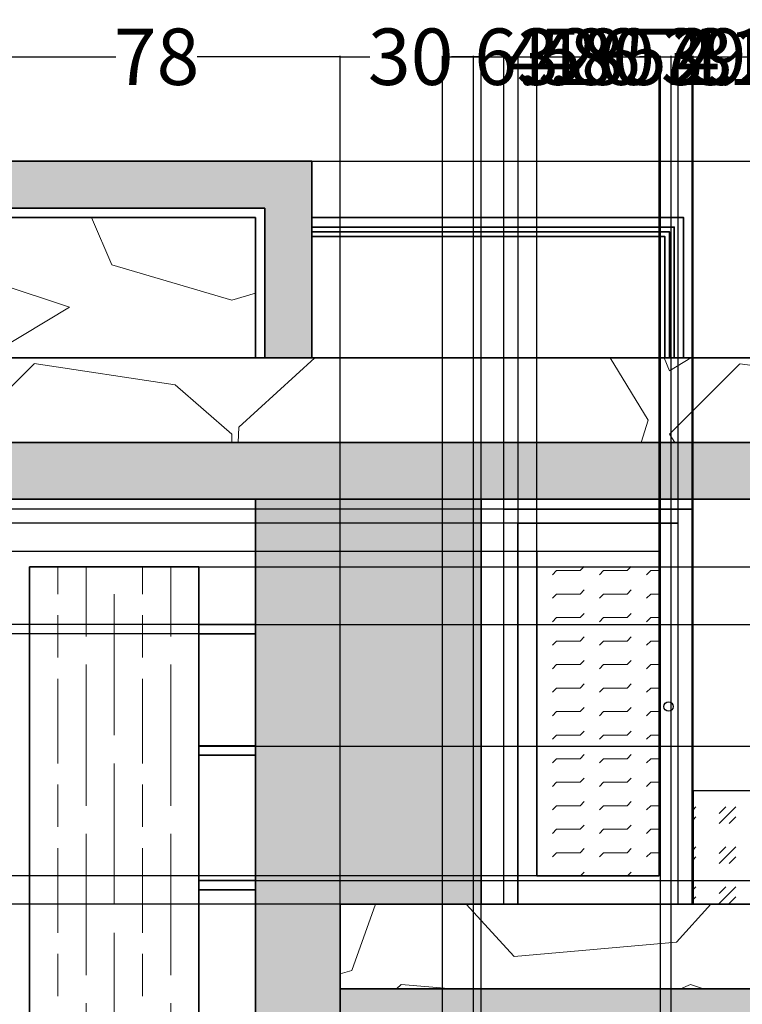
# Model space of a CAD drawing. Units: inches. Extents: x -73 to 458, y -161 to 332.
# Tile 4 of 6: x 106 to 259, y 123 to 332. Entities that reach past the tile are written whole.
import ezdxf

# ---------------------------------------------------------------- set-up
doc = ezdxf.new("R2010")
doc.units = ezdxf.units.IN
doc.header["$MEASUREMENT"] = 0
for name, color, linetype, lineweight in [('A-ANNO-DIMS', 2, 'Continuous', 18), ('A-DOOR', 4, 'Continuous', 25), ('A-ELEV', 7, 'Continuous', 35), ('A-ELEV-PATT', 8, 'Continuous', 13), ('A-GLAZ', 3, 'Continuous', 25), ('A-GLAZ-PATT', 8, 'Continuous', 13)]:
    doc.layers.add(name, color=color, linetype=linetype, lineweight=lineweight)
doc.styles.get("Standard").update_dxf_attribs({"font": 'arial.ttf'})
doc.dimstyles.get("Standard").update_dxf_attribs({"dimtxt": 12, "dimasz": 0.18, "dimexe": 0.18, "dimexo": 0.0625, "dimgap": 0.09, "dimtad": 0, "dimtih": 1, "dimtoh": 1, "dimdec": 0, "dimzin": 0, "dimdsep": 46, "dimlunit": 3, "dimtxsty": 'Standard', "dimcen": 0.09, "dimadec": 0, "dimazin": 0, "dimtfac": 1, "dimtdec": 0, "dimtofl": 0, "dimtmove": 0, "dimatfit": 3, "dimfxl": 1, "dimtolj": 1, "dimtzin": 0, "dimarcsym": 0})

# ---------------------------------------------------------------- blocks, each defined once
blk = doc.blocks.new('*U3')
blk.add_lwpolyline([(3.12, 0.01), (0.12, 0.01), (0.12, 84.01), (40.12, 84.01), (40.12, 0.01), (37.12, 0.01)])
for points in [[(37.12, 80.99), (37.12, 0.01), (3.12, 0.01), (3.12, 80.99)], [(33.12, 6.01), (33.12, 74.99), (7.12, 74.99), (7.12, 6.01)]]:
    blk.add_lwpolyline(points, close=True)
blk.add_circle((35.12, 42.01), 1)
blk = doc.blocks.new('*D6')
at = {"layer": 'A-ANNO-DIMS', "color": 0, "lineweight": -2, "transparency": 16777216}
for p, q in [((96, 260.27), (96, 324.4)), ((96.18, 324.22), (126.35, 324.22)), ((173.82, 324.22), (143.65, 324.22)), ((174, 126.13), (174, 324.4))]:
    blk.add_line(p, q, dxfattribs=at)
at = {"layer": 'A-ANNO-DIMS', "color": 0, "transparency": 16777216}
for points in [[(96.18, 324.25), (96.18, 324.19), (96, 324.22)], [(173.82, 324.25), (173.82, 324.19), (174, 324.22)]]:
    blk.add_solid(points, dxfattribs=at)
at = {"layer": 'Defpoints', "color": 0, "transparency": 16777216}
for p in [(174, 324.22), (96, 260.21), (174, 126.07)]:
    blk.add_point(p, dxfattribs=at)
at = {"layer": 'A-ANNO-DIMS', "color": 0, "transparency": 16777216, "insert": (135, 324.22), "char_height": 12, "attachment_point": 5}
blk.add_mtext('\\A1;78', dxfattribs=at)
blk = doc.blocks.new('*D7')
at = {"layer": 'A-ANNO-DIMS', "color": 0, "lineweight": -2, "transparency": 16777216}
for p, q in [((174, 126.13), (174, 324.4)), ((174.18, 324.22), (180.34, 324.22)), ((203.82, 324.22), (197.66, 324.22)), ((204, 24.13), (204, 324.4))]:
    blk.add_line(p, q, dxfattribs=at)
at = {"layer": 'A-ANNO-DIMS', "color": 0, "transparency": 16777216}
for points in [[(174.18, 324.25), (174.18, 324.19), (174, 324.22)], [(203.82, 324.25), (203.82, 324.19), (204, 324.22)]]:
    blk.add_solid(points, dxfattribs=at)
at = {"layer": 'Defpoints', "color": 0, "transparency": 16777216}
for p in [(204, 324.22), (174, 126.07), (204, 24.07)]:
    blk.add_point(p, dxfattribs=at)
at = {"layer": 'A-ANNO-DIMS', "color": 0, "transparency": 16777216, "insert": (189, 324.22), "char_height": 12, "attachment_point": 5}
blk.add_mtext('\\A1;30', dxfattribs=at)
blk = doc.blocks.new('*D8')
at = {"layer": 'A-ANNO-DIMS', "color": 0, "lineweight": -2, "transparency": 16777216}
for p, q in [((204, 24.13), (204, 324.4)), ((204.18, 324.22), (257.28, 324.22)), ((335.82, 324.22), (282.72, 324.22)), ((336, 126.13), (336, 324.4))]:
    blk.add_line(p, q, dxfattribs=at)
at = {"layer": 'A-ANNO-DIMS', "color": 0, "transparency": 16777216}
for points in [[(204.18, 324.25), (204.18, 324.19), (204, 324.22)], [(335.82, 324.25), (335.82, 324.19), (336, 324.22)]]:
    blk.add_solid(points, dxfattribs=at)
at = {"layer": 'Defpoints', "color": 0, "transparency": 16777216}
for p in [(336, 324.22), (336, 126.07), (204, 24.07)]:
    blk.add_point(p, dxfattribs=at)
at = {"layer": 'A-ANNO-DIMS', "color": 0, "transparency": 16777216, "insert": (270, 324.22), "char_height": 12, "attachment_point": 5}
blk.add_mtext('\\A1;132', dxfattribs=at)
blk = doc.blocks.new('*D25')
at = {"layer": 'A-ANNO-DIMS', "color": 0, "lineweight": -2, "transparency": 16777216}
for p, q in [((168.06, 302.02), (408.51, 302.02)), ((408.33, 301.84), (408.33, 287.33)), ((408.33, 260.39), (408.33, 274.9)), ((168.06, 260.21), (408.51, 260.21))]:
    blk.add_line(p, q, dxfattribs=at)
at = {"layer": 'A-ANNO-DIMS', "color": 0, "transparency": 16777216}
for points in [[(408.3, 301.84), (408.36, 301.84), (408.33, 302.02)], [(408.3, 260.39), (408.36, 260.39), (408.33, 260.21)]]:
    blk.add_solid(points, dxfattribs=at)
at = {"layer": 'Defpoints', "color": 0, "transparency": 16777216}
for p in [(168, 302.02), (408.33, 302.02), (168, 260.21)]:
    blk.add_point(p, dxfattribs=at)
at = {"layer": 'A-ANNO-DIMS', "color": 0, "transparency": 16777216, "insert": (408.33, 281.11), "char_height": 12, "attachment_point": 5}
blk.add_mtext('\\A1;41.814', dxfattribs=at)
blk = doc.blocks.new('*D42')
at = {"layer": 'A-ANNO-DIMS', "color": 0, "lineweight": -2, "transparency": 16777216}
for p, q in [((144.06, 149.14), (408.51, 149.14)), ((408.33, 148.96), (408.33, 140.32)), ((408.33, 119.24), (408.33, 127.88)), ((144.06, 119.06), (408.51, 119.06))]:
    blk.add_line(p, q, dxfattribs=at)
at = {"layer": 'A-ANNO-DIMS', "color": 0, "transparency": 16777216}
for points in [[(408.3, 148.96), (408.36, 148.96), (408.33, 149.14)], [(408.3, 119.24), (408.36, 119.24), (408.33, 119.06)]]:
    blk.add_solid(points, dxfattribs=at)
at = {"layer": 'Defpoints', "color": 0, "transparency": 16777216}
for p in [(144, 149.14), (408.33, 149.14), (144, 119.06)]:
    blk.add_point(p, dxfattribs=at)
at = {"layer": 'A-ANNO-DIMS', "color": 0, "transparency": 16777216, "insert": (408.33, 134.1), "char_height": 12, "attachment_point": 5}
blk.add_mtext('\\A1;30.08', dxfattribs=at)
blk = doc.blocks.new('*D43')
at = {"layer": 'A-ANNO-DIMS', "color": 0, "lineweight": -2, "transparency": 16777216}
for p, q in [((144.06, 177.7), (408.51, 177.7)), ((408.33, 177.52), (408.33, 169.64)), ((408.33, 149.32), (408.33, 157.2)), ((144.06, 149.14), (408.51, 149.14))]:
    blk.add_line(p, q, dxfattribs=at)
at = {"layer": 'A-ANNO-DIMS', "color": 0, "transparency": 16777216}
for points in [[(408.3, 177.52), (408.36, 177.52), (408.33, 177.7)], [(408.3, 149.32), (408.36, 149.32), (408.33, 149.14)]]:
    blk.add_solid(points, dxfattribs=at)
at = {"layer": 'Defpoints', "color": 0, "transparency": 16777216}
for p in [(144, 177.7), (408.33, 177.7), (144, 149.14)]:
    blk.add_point(p, dxfattribs=at)
at = {"layer": 'A-ANNO-DIMS', "color": 0, "transparency": 16777216, "insert": (408.33, 163.42), "char_height": 12, "attachment_point": 5}
blk.add_mtext('\\A1;28.57', dxfattribs=at)
blk = doc.blocks.new('*D44')
at = {"layer": 'A-ANNO-DIMS', "color": 0, "lineweight": -2, "transparency": 16777216}
for p, q in [((144.06, 203.54), (408.51, 203.54)), ((408.33, 203.36), (408.33, 196.84)), ((408.33, 177.88), (408.33, 184.4)), ((144.06, 177.7), (408.51, 177.7))]:
    blk.add_line(p, q, dxfattribs=at)
at = {"layer": 'A-ANNO-DIMS', "color": 0, "transparency": 16777216}
for points in [[(408.3, 203.36), (408.36, 203.36), (408.33, 203.54)], [(408.3, 177.88), (408.36, 177.88), (408.33, 177.7)]]:
    blk.add_solid(points, dxfattribs=at)
at = {"layer": 'Defpoints', "color": 0, "transparency": 16777216}
for p in [(144, 203.54), (408.33, 203.54), (144, 177.7)]:
    blk.add_point(p, dxfattribs=at)
at = {"layer": 'A-ANNO-DIMS', "color": 0, "transparency": 16777216, "insert": (408.33, 190.62), "char_height": 12, "attachment_point": 5}
blk.add_mtext('\\A1;25.83', dxfattribs=at)
blk = doc.blocks.new('*D45')
at = {"layer": 'A-ANNO-DIMS', "color": 0, "lineweight": -2, "transparency": 16777216}
for p, q in [((144.06, 215.8), (408.51, 215.8)), ((408.33, 215.8), (408.33, 215.98)), ((408.33, 215.98), (408.51, 215.98)), ((408.33, 203.72), (408.33, 215.62)), ((144.06, 203.54), (408.51, 203.54))]:
    blk.add_line(p, q, dxfattribs=at)
at = {"layer": 'A-ANNO-DIMS', "color": 0, "transparency": 16777216}
for points in [[(408.3, 215.62), (408.36, 215.62), (408.33, 215.8)], [(408.3, 203.72), (408.36, 203.72), (408.33, 203.54)]]:
    blk.add_solid(points, dxfattribs=at)
at = {"layer": 'Defpoints', "color": 0, "transparency": 16777216}
for p in [(144, 215.8), (408.33, 215.8), (144, 203.54)]:
    blk.add_point(p, dxfattribs=at)
at = {"layer": 'A-ANNO-DIMS', "color": 0, "transparency": 16777216, "insert": (432.98, 215.98), "char_height": 12, "attachment_point": 5}
blk.add_mtext('\\A1;12.265', dxfattribs=at)
blk = doc.blocks.new('*D46')
at = {"layer": 'A-ANNO-DIMS', "color": 0, "lineweight": -2, "transparency": 16777216}
for p, q in [((156.06, 230.21), (408.51, 230.21)), ((408.33, 230.03), (408.33, 229.22)), ((144.06, 215.8), (408.51, 215.8)), ((408.33, 215.98), (408.33, 216.79))]:
    blk.add_line(p, q, dxfattribs=at)
at = {"layer": 'A-ANNO-DIMS', "color": 0, "transparency": 16777216}
for points in [[(408.3, 230.03), (408.36, 230.03), (408.33, 230.21)], [(408.3, 215.98), (408.36, 215.98), (408.33, 215.8)]]:
    blk.add_solid(points, dxfattribs=at)
at = {"layer": 'Defpoints', "color": 0, "transparency": 16777216}
for p in [(156, 230.21), (408.33, 230.21), (144, 215.8)]:
    blk.add_point(p, dxfattribs=at)
at = {"layer": 'A-ANNO-DIMS', "color": 0, "transparency": 16777216, "insert": (408.33, 223), "char_height": 12, "attachment_point": 5}
blk.add_mtext('\\A1;14.406', dxfattribs=at)
blk = doc.blocks.new('*D47')
at = {"layer": 'A-ANNO-DIMS', "color": 0, "lineweight": -2, "transparency": 16777216}
for p, q in [((143.94, 203.54), (-41.78, 203.54)), ((-41.6, 203.36), (-41.6, 201.74)), ((143.94, 201.56), (-41.78, 201.56)), ((-41.6, 201.38), (-41.78, 201.38)), ((-41.6, 201.56), (-41.6, 201.38))]:
    blk.add_line(p, q, dxfattribs=at)
at = {"layer": 'A-ANNO-DIMS', "color": 0, "transparency": 16777216}
for points in [[(-41.63, 203.36), (-41.57, 203.36), (-41.6, 203.54)], [(-41.63, 201.74), (-41.57, 201.74), (-41.6, 201.56)]]:
    blk.add_solid(points, dxfattribs=at)
at = {"layer": 'Defpoints', "color": 0, "transparency": 16777216}
for p in [(144, 203.54), (-41.6, 201.56), (144, 201.56)]:
    blk.add_point(p, dxfattribs=at)
at = {"layer": 'A-ANNO-DIMS', "color": 0, "transparency": 16777216, "insert": (-56.91, 201.38), "char_height": 12, "attachment_point": 5}
blk.add_mtext('\\A1;1.98', dxfattribs=at)
blk = doc.blocks.new('*D48')
at = {"layer": 'A-ANNO-DIMS', "color": 0, "lineweight": -2, "transparency": 16777216}
for p, q in [((204, 144.13), (204, 324.4)), ((204.18, 324.22), (208.63, 324.22)), ((208.81, 144.14), (208.81, 324.4)), ((208.81, 324.22), (208.99, 324.22))]:
    blk.add_line(p, q, dxfattribs=at)
at = {"layer": 'A-ANNO-DIMS', "color": 0, "transparency": 16777216}
for points in [[(204.18, 324.25), (204.18, 324.19), (204, 324.22)], [(208.63, 324.25), (208.63, 324.19), (208.81, 324.22)]]:
    blk.add_solid(points, dxfattribs=at)
at = {"layer": 'Defpoints', "color": 0, "transparency": 16777216}
for p in [(208.81, 324.22), (204, 144.07), (208.81, 144.08)]:
    blk.add_point(p, dxfattribs=at)
at = {"layer": 'A-ANNO-DIMS', "color": 0, "transparency": 16777216, "insert": (229.56, 324.22), "char_height": 12, "attachment_point": 5}
blk.add_mtext('\\A1;4.807', dxfattribs=at)
blk = doc.blocks.new('*D49')
at = {"layer": 'A-ANNO-DIMS', "color": 0, "lineweight": -2, "transparency": 16777216}
for p, q in [((208.81, 144.14), (208.81, 324.4)), ((208.99, 324.22), (211.63, 324.22)), ((211.81, 144.14), (211.81, 324.4)), ((211.81, 324.22), (211.99, 324.22))]:
    blk.add_line(p, q, dxfattribs=at)
at = {"layer": 'A-ANNO-DIMS', "color": 0, "transparency": 16777216}
for points in [[(208.99, 324.25), (208.99, 324.19), (208.81, 324.22)], [(211.63, 324.25), (211.63, 324.19), (211.81, 324.22)]]:
    blk.add_solid(points, dxfattribs=at)
at = {"layer": 'Defpoints', "color": 0, "transparency": 16777216}
for p in [(211.81, 324.22), (208.81, 144.08), (211.81, 144.08)]:
    blk.add_point(p, dxfattribs=at)
at = {"layer": 'A-ANNO-DIMS', "color": 0, "transparency": 16777216, "insert": (216, 324.22), "char_height": 12, "attachment_point": 5}
blk.add_mtext('\\A1;3', dxfattribs=at)
blk = doc.blocks.new('*D50')
at = {"layer": 'A-ANNO-DIMS', "color": 0, "lineweight": -2, "transparency": 16777216}
for p, q in [((211.81, 144.14), (211.81, 324.4)), ((211.99, 324.22), (215.63, 324.22)), ((215.81, 150.14), (215.81, 324.4)), ((215.81, 324.22), (215.99, 324.22))]:
    blk.add_line(p, q, dxfattribs=at)
at = {"layer": 'A-ANNO-DIMS', "color": 0, "transparency": 16777216}
for points in [[(211.99, 324.25), (211.99, 324.19), (211.81, 324.22)], [(215.63, 324.25), (215.63, 324.19), (215.81, 324.22)]]:
    blk.add_solid(points, dxfattribs=at)
at = {"layer": 'Defpoints', "color": 0, "transparency": 16777216}
for p in [(215.81, 324.22), (215.81, 150.08), (211.81, 144.08)]:
    blk.add_point(p, dxfattribs=at)
at = {"layer": 'A-ANNO-DIMS', "color": 0, "transparency": 16777216, "insert": (220.23, 324.22), "char_height": 12, "attachment_point": 5}
blk.add_mtext('\\A1;4', dxfattribs=at)
blk = doc.blocks.new('*D51')
at = {"layer": 'A-ANNO-DIMS', "color": 0, "lineweight": -2, "transparency": 16777216}
for p, q in [((215.81, 150.14), (215.81, 324.4)), ((215.99, 324.22), (220.02, 324.22)), ((241.63, 324.22), (237.59, 324.22)), ((241.81, 150.14), (241.81, 324.4))]:
    blk.add_line(p, q, dxfattribs=at)
at = {"layer": 'A-ANNO-DIMS', "color": 0, "transparency": 16777216}
for points in [[(215.99, 324.25), (215.99, 324.19), (215.81, 324.22)], [(241.63, 324.25), (241.63, 324.19), (241.81, 324.22)]]:
    blk.add_solid(points, dxfattribs=at)
at = {"layer": 'Defpoints', "color": 0, "transparency": 16777216}
for p in [(241.81, 324.22), (215.81, 150.08), (241.81, 150.08)]:
    blk.add_point(p, dxfattribs=at)
at = {"layer": 'A-ANNO-DIMS', "color": 0, "transparency": 16777216, "insert": (228.81, 324.22), "char_height": 12, "attachment_point": 5}
blk.add_mtext('\\A1;26', dxfattribs=at)
blk = doc.blocks.new('*D52')
at = {"layer": 'A-ANNO-DIMS', "color": 0, "lineweight": -2, "transparency": 16777216}
for p, q in [((241.81, 150.14), (241.81, 324.4)), ((241.99, 324.22), (245.63, 324.22)), ((245.81, 144.14), (245.81, 324.4)), ((245.81, 324.22), (245.99, 324.22))]:
    blk.add_line(p, q, dxfattribs=at)
at = {"layer": 'A-ANNO-DIMS', "color": 0, "transparency": 16777216}
for points in [[(241.99, 324.25), (241.99, 324.19), (241.81, 324.22)], [(245.63, 324.25), (245.63, 324.19), (245.81, 324.22)]]:
    blk.add_solid(points, dxfattribs=at)
at = {"layer": 'Defpoints', "color": 0, "transparency": 16777216}
for p in [(245.81, 324.22), (241.81, 150.08), (245.81, 144.08)]:
    blk.add_point(p, dxfattribs=at)
at = {"layer": 'A-ANNO-DIMS', "color": 0, "transparency": 16777216, "insert": (250.23, 324.22), "char_height": 12, "attachment_point": 5}
blk.add_mtext('\\A1;4', dxfattribs=at)
blk = doc.blocks.new('*D53')
at = {"layer": 'A-ANNO-DIMS', "color": 0, "lineweight": -2, "transparency": 16777216}
for p, q in [((245.81, 144.14), (245.81, 324.4)), ((245.99, 324.22), (248.63, 324.22)), ((248.81, 144.14), (248.81, 324.4)), ((248.81, 324.22), (248.99, 324.22))]:
    blk.add_line(p, q, dxfattribs=at)
at = {"layer": 'A-ANNO-DIMS', "color": 0, "transparency": 16777216}
for points in [[(245.99, 324.25), (245.99, 324.19), (245.81, 324.22)], [(248.63, 324.25), (248.63, 324.19), (248.81, 324.22)]]:
    blk.add_solid(points, dxfattribs=at)
at = {"layer": 'Defpoints', "color": 0, "transparency": 16777216}
for p in [(248.81, 324.22), (245.81, 144.08), (248.81, 144.08)]:
    blk.add_point(p, dxfattribs=at)
at = {"layer": 'A-ANNO-DIMS', "color": 0, "transparency": 16777216, "insert": (253, 324.22), "char_height": 12, "attachment_point": 5}
blk.add_mtext('\\A1;3', dxfattribs=at)
blk = doc.blocks.new('*D54')
at = {"layer": 'A-ANNO-DIMS', "color": 0, "lineweight": -2, "transparency": 16777216}
for p, q in [((249, 168.25), (249, 324.4)), ((249.18, 324.22), (262.15, 324.22)), ((262.33, 168.25), (262.33, 324.4)), ((262.33, 324.22), (262.51, 324.22))]:
    blk.add_line(p, q, dxfattribs=at)
at = {"layer": 'A-ANNO-DIMS', "color": 0, "transparency": 16777216}
for points in [[(249.18, 324.25), (249.18, 324.19), (249, 324.22)], [(262.15, 324.25), (262.15, 324.19), (262.33, 324.22)]]:
    blk.add_solid(points, dxfattribs=at)
at = {"layer": 'Defpoints', "color": 0, "transparency": 16777216}
for p in [(262.33, 324.22), (249, 168.19), (262.33, 168.19)]:
    blk.add_point(p, dxfattribs=at)
at = {"layer": 'A-ANNO-DIMS', "color": 0, "transparency": 16777216, "insert": (282.28, 324.22), "char_height": 12, "attachment_point": 5}
blk.add_mtext('\\A1;13.33', dxfattribs=at)
blk = doc.blocks.new('*D61')
at = {"layer": 'A-ANNO-DIMS', "color": 0, "lineweight": -2, "transparency": 16777216}
for p, q in [((241.74, 150.08), (-41.78, 150.08)), ((-41.6, 150.08), (-41.6, 150.26)), ((-41.6, 150.26), (-41.42, 150.26)), ((-41.6, 144.26), (-41.6, 149.9)), ((248.74, 144.08), (-41.78, 144.08))]:
    blk.add_line(p, q, dxfattribs=at)
at = {"layer": 'A-ANNO-DIMS', "color": 0, "transparency": 16777216}
for points in [[(-41.63, 149.9), (-41.57, 149.9), (-41.6, 150.08)], [(-41.63, 144.26), (-41.57, 144.26), (-41.6, 144.08)]]:
    blk.add_solid(points, dxfattribs=at)
at = {"layer": 'Defpoints', "color": 0, "transparency": 16777216}
for p in [(-41.6, 150.08), (241.81, 150.08), (248.81, 144.08)]:
    blk.add_point(p, dxfattribs=at)
at = {"layer": 'A-ANNO-DIMS', "color": 0, "transparency": 16777216, "insert": (-37.37, 150.26), "char_height": 12, "attachment_point": 5}
blk.add_mtext('\\A1;6', dxfattribs=at)
blk = doc.blocks.new('*D62')
at = {"layer": 'A-ANNO-DIMS', "color": 0, "lineweight": -2, "transparency": 16777216}
for p, q in [((241.74, 219.06), (-41.78, 219.06)), ((-41.6, 218.88), (-41.6, 190.78)), ((-41.6, 150.26), (-41.6, 178.35)), ((241.74, 150.08), (-41.78, 150.08))]:
    blk.add_line(p, q, dxfattribs=at)
at = {"layer": 'A-ANNO-DIMS', "color": 0, "transparency": 16777216}
for points in [[(-41.63, 218.88), (-41.57, 218.88), (-41.6, 219.06)], [(-41.63, 150.26), (-41.57, 150.26), (-41.6, 150.08)]]:
    blk.add_solid(points, dxfattribs=at)
at = {"layer": 'Defpoints', "color": 0, "transparency": 16777216}
for p in [(-41.6, 219.06), (241.81, 219.06), (241.81, 150.08)]:
    blk.add_point(p, dxfattribs=at)
at = {"layer": 'A-ANNO-DIMS', "color": 0, "transparency": 16777216, "insert": (-41.6, 184.57), "char_height": 12, "attachment_point": 5}
blk.add_mtext('\\A1;68.98', dxfattribs=at)
blk = doc.blocks.new('*D63')
at = {"layer": 'A-ANNO-DIMS', "color": 0, "lineweight": -2, "transparency": 16777216}
for p, q in [((245.74, 225.06), (-41.78, 225.06)), ((-41.6, 225.06), (-41.6, 225.24)), ((-41.6, 225.24), (-41.42, 225.24)), ((-41.6, 219.24), (-41.6, 224.88)), ((241.74, 219.06), (-41.78, 219.06))]:
    blk.add_line(p, q, dxfattribs=at)
at = {"layer": 'A-ANNO-DIMS', "color": 0, "transparency": 16777216}
for points in [[(-41.63, 224.88), (-41.57, 224.88), (-41.6, 225.06)], [(-41.63, 219.24), (-41.57, 219.24), (-41.6, 219.06)]]:
    blk.add_solid(points, dxfattribs=at)
at = {"layer": 'Defpoints', "color": 0, "transparency": 16777216}
for p in [(-41.6, 225.06), (245.81, 225.06), (241.81, 219.06)]:
    blk.add_point(p, dxfattribs=at)
at = {"layer": 'A-ANNO-DIMS', "color": 0, "transparency": 16777216, "insert": (-37.37, 225.24), "char_height": 12, "attachment_point": 5}
blk.add_mtext('\\A1;6', dxfattribs=at)
blk = doc.blocks.new('*D64')
at = {"layer": 'A-ANNO-DIMS', "color": 0, "lineweight": -2, "transparency": 16777216}
for p, q in [((-41.6, 228.08), (-41.6, 228.26)), ((-41.6, 228.26), (-41.42, 228.26)), ((248.74, 228.08), (-41.78, 228.08)), ((-41.6, 225.24), (-41.6, 227.9)), ((245.74, 225.06), (-41.78, 225.06))]:
    blk.add_line(p, q, dxfattribs=at)
at = {"layer": 'A-ANNO-DIMS', "color": 0, "transparency": 16777216}
for points in [[(-41.63, 227.9), (-41.57, 227.9), (-41.6, 228.08)], [(-41.63, 225.24), (-41.57, 225.24), (-41.6, 225.06)]]:
    blk.add_solid(points, dxfattribs=at)
at = {"layer": 'Defpoints', "color": 0, "transparency": 16777216}
for p in [(-41.6, 228.08), (248.81, 228.08), (245.81, 225.06)]:
    blk.add_point(p, dxfattribs=at)
at = {"layer": 'A-ANNO-DIMS', "color": 0, "transparency": 16777216, "insert": (-21.09, 228.26), "char_height": 12, "attachment_point": 5}
blk.add_mtext('\\A1;3.023', dxfattribs=at)
blk = doc.blocks.new('*D71')
at = {"layer": 'A-ANNO-DIMS', "color": 0, "lineweight": -2, "transparency": 16777216}
for p, q in [((195.77, -5.87), (195.77, 324.4)), ((195.95, 324.22), (202.17, 324.22)), ((202.35, -5.87), (202.35, 324.4)), ((202.35, 324.22), (202.53, 324.22))]:
    blk.add_line(p, q, dxfattribs=at)
at = {"layer": 'A-ANNO-DIMS', "color": 0, "transparency": 16777216}
for points in [[(195.95, 324.25), (195.95, 324.19), (195.77, 324.22)], [(202.17, 324.25), (202.17, 324.19), (202.35, 324.22)]]:
    blk.add_solid(points, dxfattribs=at)
at = {"layer": 'Defpoints', "color": 0, "transparency": 16777216}
for p in [(202.35, 324.22), (195.77, -5.93), (202.35, -5.93)]:
    blk.add_point(p, dxfattribs=at)
at = {"layer": 'A-ANNO-DIMS', "color": 0, "transparency": 16777216, "insert": (222.95, 324.22), "char_height": 12, "attachment_point": 5}
blk.add_mtext('\\A1;6.585', dxfattribs=at)
blk = doc.blocks.new('*D72')
at = {"layer": 'A-ANNO-DIMS', "color": 0, "lineweight": -2, "transparency": 16777216}
for p, q in [((202.35, -5.87), (202.35, 324.4)), ((202.53, 324.22), (241.93, 324.22)), ((242.11, -5.87), (242.11, 324.4)), ((242.11, 324.22), (242.29, 324.22))]:
    blk.add_line(p, q, dxfattribs=at)
at = {"layer": 'A-ANNO-DIMS', "color": 0, "transparency": 16777216}
for points in [[(202.53, 324.25), (202.53, 324.19), (202.35, 324.22)], [(241.93, 324.25), (241.93, 324.19), (242.11, 324.22)]]:
    blk.add_solid(points, dxfattribs=at)
at = {"layer": 'Defpoints', "color": 0, "transparency": 16777216}
for p in [(242.11, 324.22), (202.35, -5.93), (242.11, -5.93)]:
    blk.add_point(p, dxfattribs=at)
at = {"layer": 'A-ANNO-DIMS', "color": 0, "transparency": 16777216, "insert": (262.62, 324.22), "char_height": 12, "attachment_point": 5}
blk.add_mtext('\\A1;39.76', dxfattribs=at)
blk = doc.blocks.new('*D73')
at = {"layer": 'A-ANNO-DIMS', "color": 0, "lineweight": -2, "transparency": 16777216}
for p, q in [((242.11, -5.87), (242.11, 324.4)), ((242.29, 324.22), (244.17, 324.22)), ((244.35, -5.87), (244.35, 324.4)), ((244.35, 324.22), (244.53, 324.22))]:
    blk.add_line(p, q, dxfattribs=at)
at = {"layer": 'A-ANNO-DIMS', "color": 0, "transparency": 16777216}
for points in [[(242.29, 324.25), (242.29, 324.19), (242.11, 324.22)], [(244.17, 324.25), (244.17, 324.19), (244.35, 324.22)]]:
    blk.add_solid(points, dxfattribs=at)
at = {"layer": 'Defpoints', "color": 0, "transparency": 16777216}
for p in [(244.35, 324.22), (242.11, -5.93), (244.35, -5.93)]:
    blk.add_point(p, dxfattribs=at)
at = {"layer": 'A-ANNO-DIMS', "color": 0, "transparency": 16777216, "insert": (264.95, 324.22), "char_height": 12, "attachment_point": 5}
blk.add_mtext('\\A1;2.244', dxfattribs=at)
blk = doc.blocks.new('*D74')
at = {"layer": 'A-ANNO-DIMS', "color": 0, "lineweight": -2, "transparency": 16777216}
for p, q in [((244.35, -5.87), (244.35, 324.4)), ((244.53, 324.22), (277.93, 324.22)), ((278.11, -5.87), (278.11, 324.4)), ((278.11, 324.22), (278.29, 324.22))]:
    blk.add_line(p, q, dxfattribs=at)
at = {"layer": 'A-ANNO-DIMS', "color": 0, "transparency": 16777216}
for points in [[(244.53, 324.25), (244.53, 324.19), (244.35, 324.22)], [(277.93, 324.25), (277.93, 324.19), (278.11, 324.22)]]:
    blk.add_solid(points, dxfattribs=at)
at = {"layer": 'Defpoints', "color": 0, "transparency": 16777216}
for p in [(278.11, 324.22), (244.35, -5.93), (278.11, -5.93)]:
    blk.add_point(p, dxfattribs=at)
at = {"layer": 'A-ANNO-DIMS', "color": 0, "transparency": 16777216, "insert": (303.28, 324.22), "char_height": 12, "attachment_point": 5}
blk.add_mtext('\\A1;33.756', dxfattribs=at)

msp = doc.modelspace()

# ---------------------------------------------------------------- hatches: boundary and pattern name
at = {"layer": 'A-ELEV-PATT'}
h = msp.add_hatch(color=256, dxfattribs=at)
h.dxf.hatch_style = 1
h.paths.add_polyline_path([(167.9979, 302.0202), (155.9979, 302.0202), (95.9979, 302.0202), (23.9979, 302.0202), (23.9979, -113.9335), (33.9979, -113.9335), (33.9979, 292.0202), (95.9979, 292.0202), (157.9979, 292.0202), (157.9979, 260.2059), (167.9979, 260.2059), (167.9979, 290.0202)])
h.paths.add_polyline_path([(335.9979, 242.2059), (323.9979, 242.2059), (95.9979, 242.2059), (95.9979, 234.0665), (95.9979, 230.2059), (323.9979, 230.2059), (335.9979, 230.2059)])
h.paths.add_polyline_path([(335.9979, 126.0665), (323.9979, 126.0665), (173.9979, 126.0665), (173.9979, 114.0665), (323.9979, 114.0665), (335.9979, 114.0665)])
h.paths.add_polyline_path([(335.9979, 6.0665), (323.9979, 6.0665), (95.9979, 6.0665), (95.9979, -5.9335), (323.9979, -5.9335), (335.9979, -5.9335)])
h = msp.add_hatch(dxfattribs=at)
h.set_pattern_fill('GRAVEL', color=256, scale=150)
h.paths.add_polyline_path([(95.9979, 234.0665), (95.9979, 260.2059), (155.9979, 260.2059), (155.9979, 290.0202), (95.9979, 290.0202), (55.9979, 290.0202), (55.9979, -113.9335), (95.9979, -113.9335), (95.9979, 24.0665), (95.9979, 54.0267)])
h.paths.add_polyline_path([(323.9979, 144.0665), (248.9979, 144.0665), (173.9979, 144.0665), (173.9979, 126.0665), (323.9979, 126.0665)])
h.paths.add_polyline_path([(323.9979, 24.0665), (248.9979, 24.0665), (155.9979, 24.0665), (155.9979, 6.0665), (323.9979, 6.0665)])
h.paths.add_polyline_path([(323.9979, 260.2059), (95.9979, 260.2059), (95.9979, 242.2059), (323.9979, 242.2059)])
h.paths.add_polyline_path([(155.9979, 24.0665), (95.9979, 24.0665), (95.9979, 6.0665), (155.9979, 6.0665)], flags=17)
h = msp.add_hatch(color=256, dxfattribs=at)
h.dxf.hatch_style = 1
h.paths.add_polyline_path([(195.7666, -5.9335), (155.3839, -5.9335), (155.3839, -113.9335), (195.7666, -113.9335)])
h.paths.add_polyline_path([(323.9979, -5.9335), (284.4845, -5.9335), (284.4845, -113.9335), (323.9979, -113.9335)])
h.paths.add_polyline_path([(203.9979, 114.0665), (173.9979, 114.0665), (173.9979, 144.0665), (203.9979, 144.0665), (203.9979, 230.2059), (155.9979, 230.2059), (155.9979, 24.0665), (203.9979, 24.0665)])
h = msp.add_hatch(dxfattribs=at)
h.set_pattern_fill('FLEX', color=256, scale=20)
h.paths.add_polyline_path([(241.805, 219.0563), (215.805, 219.0563), (215.805, 150.0793), (241.805, 150.0793)])
h.paths.add_polyline_path([(241.805, 99.0563), (215.805, 99.0563), (215.805, 30.0793), (241.805, 30.0793)])
h.paths.add_polyline_path([(138.915, -38.9437), (112.915, -38.9437), (112.915, -107.9207), (138.915, -107.9207)])
h = msp.add_hatch(dxfattribs=at)
h.set_pattern_fill('GOST_WOOD', color=256, scale=3)
h.set_pattern_definition([(90, (0, 0), (18, -1e-15), [30, -6]), (90, (6, -6), (18, -1e-15), [18, -4.5, 9, -4.5]), (90, (12, -15), (18, -1e-15), [30, -6])])
h.paths.add_polyline_path([(143.9979, 215.8003), (107.9979, 215.8003), (107.9979, 54.0267), (143.9979, 54.0267)])

# ---------------------------------------------------------------- linework, layer by layer
at = {"layer": 'A-ELEV'}
for p, q in [((167.9979, 260.2059), (167.9979, 290.0202)), ((323.9979, 260.2059), (95.9979, 260.2059)), ((246.9957, 260.2059), (167.9979, 260.2059)), ((323.9979, 242.2059), (95.9979, 242.2059)), ((323.9979, 230.2059), (95.9979, 230.2059)), ((155.9979, 6.0665), (155.9979, 230.2059)), ((203.9979, 144.0665), (203.9979, 230.2059)), ((107.9979, 215.8003), (107.9979, 54.0267)), ((143.9979, 215.8003), (107.9979, 215.8003)), ((143.9979, 54.0267), (143.9979, 215.8003)), ((323.9979, 144.0665), (173.9979, 144.0665)), ((173.9979, 144.0665), (173.9979, 114.0665)), ((323.9979, 126.0665), (173.9979, 126.0665))]:
    msp.add_line(p, q, dxfattribs=at)
for points in [[(167.9979, 260.2059), (167.9979, 302.0202), (155.9979, 302.0202), (95.9979, 302.0202), (23.9979, 302.0202), (23.9979, -113.9335)], [(157.9979, 260.2059), (157.9979, 292.0202), (95.9979, 292.0202), (33.9979, 292.0202), (33.9979, -113.9335)], [(155.9979, 260.2059), (155.9979, 290.0202), (95.9979, 290.0202), (35.9979, 290.0202), (35.9979, -113.9335)], [(167.9979, 290.0202), (246.9957, 290.0202), (246.9957, 260.2059)], [(167.9979, 288.0202), (244.9957, 288.0202), (244.9957, 260.2059)], [(167.9979, 287.0202), (243.9957, 287.0202), (243.9957, 260.2059)], [(167.9979, 286.0202), (242.9957, 286.0202), (242.9957, 260.2059)]]:
    msp.add_lwpolyline(points, dxfattribs=at)
for points in [[(143.9979, 203.5354), (155.9979, 203.5354), (155.9979, 201.5578), (143.9979, 201.5578)], [(143.9979, 177.7045), (155.9979, 177.7045), (155.9979, 175.727), (143.9979, 175.727)], [(143.9979, 149.136), (155.9979, 149.136), (155.9979, 147.1585), (143.9979, 147.1585)]]:
    msp.add_lwpolyline(points, close=True, dxfattribs=at)
at = {"layer": 'A-GLAZ'}
msp.add_lwpolyline([(248.9979, 144.0665), (323.9979, 144.0665), (323.9979, 168.1912), (248.9979, 168.1912)], close=True, dxfattribs=at)
at = {"layer": 'A-GLAZ-PATT'}
for p, q in [((248.9979, 164.145), (249.6087, 164.7559)), ((254.5584, 161.2203), (258.094, 164.7559)), ((254.5584, 163.3417), (255.9727, 164.7559)), ((248.9979, 162.0237), (249.6087, 162.6346)), ((256.6798, 161.2203), (258.094, 162.6346)), ((248.9979, 155.6598), (249.6087, 156.2706)), ((254.5584, 152.7351), (258.094, 156.2706)), ((254.5584, 154.8564), (255.9727, 156.2706)), ((248.9979, 153.5384), (249.6087, 154.1493)), ((256.6798, 152.7351), (258.094, 154.1493)), ((248.9979, 147.1745), (249.6087, 147.7853)), ((254.5584, 144.2498), (258.094, 147.7853)), ((254.5584, 146.3711), (255.9727, 147.7853)), ((248.9979, 145.0532), (249.6087, 145.664)), ((256.6798, 144.2498), (258.094, 145.664))]:
    msp.add_line(p, q, dxfattribs=at)

# ---------------------------------------------------------------- block references
at = {"layer": 'A-DOOR'}
msp.add_blockref('*U3', (208.6813, 144.0665), dxfattribs=at)

# ---------------------------------------------------------------- dimensions: what is measured, and where the dimension line sits
at = {"layer": 'A-ANNO-DIMS'}
for base, p1, p2, override, picture, middle in [((173.9979, 324.2202), (95.9979, 260.2059), (173.9979, 126.0665), {"dimdec": 0, "dimlfac": 1, "dimrnd": 0, "dimzin": 0, "dimdsep": 46, "dimlunit": 2}, '*D6', (134.9979, 324.2202)), ((203.9979, 324.2202), (173.9979, 126.0665), (203.9979, 24.0665), {"dimdec": 0, "dimlfac": 1, "dimrnd": 0, "dimzin": 0, "dimdsep": 46, "dimlunit": 2}, '*D7', (188.9979, 324.2202)), ((202.3513, 324.2202), (195.7666, -5.9335), (202.3513, -5.9335), {"dimdec": 3, "dimlfac": 1, "dimrnd": 0, "dimzin": 0, "dimdsep": 46, "dimlunit": 2}, '*D71', (222.946, 324.2202)), ((242.1074, 324.2202), (202.3513, -5.9335), (242.1074, -5.9335), {"dimdec": 2, "dimlfac": 1, "dimrnd": 0, "dimzin": 0, "dimdsep": 46, "dimlunit": 2}, '*D72', (262.6161, 324.2202)), ((335.9979, 324.2202), (203.9979, 24.0665), (335.9979, 126.0665), {"dimdec": 0, "dimlfac": 1, "dimrnd": 0, "dimzin": 0, "dimdsep": 46, "dimlunit": 2}, '*D8', (269.9979, 324.2202)), ((208.805, 324.2202), (203.9979, 144.0665), (208.805, 144.0793), {"dimdec": 3, "dimlfac": 1, "dimrnd": 0, "dimzin": 0, "dimdsep": 46, "dimlunit": 2}, '*D48', (229.5634, 324.2202)), ((211.805, 324.2202), (208.805, 144.0793), (211.805, 144.0793), {"dimdec": 0, "dimlfac": 1, "dimrnd": 0, "dimzin": 0, "dimdsep": 46, "dimlunit": 2}, '*D49', (216.0041, 324.2202)), ((215.805, 324.2202), (211.805, 144.0793), (215.805, 150.0793), {"dimdec": 0, "dimlfac": 1, "dimrnd": 0, "dimzin": 0, "dimdsep": 46, "dimlunit": 2}, '*D50', (220.2251, 324.2202)), ((241.805, 324.2202), (215.805, 150.0793), (241.805, 150.0793), {"dimdec": 0, "dimlfac": 1, "dimrnd": 0, "dimzin": 0, "dimdsep": 46, "dimlunit": 2}, '*D51', (228.805, 324.2202)), ((245.805, 324.2202), (241.805, 150.0793), (245.805, 144.0793), {"dimdec": 0, "dimlfac": 1, "dimrnd": 0, "dimzin": 0, "dimdsep": 46, "dimlunit": 2}, '*D52', (250.2251, 324.2202)), ((244.3513, 324.2202), (242.1074, -5.9335), (244.3513, -5.9335), {"dimdec": 3, "dimlfac": 1, "dimrnd": 0, "dimzin": 0, "dimdsep": 46, "dimlunit": 2}, '*D73', (264.946, 324.2202)), ((278.1074, 324.2202), (244.3513, -5.9335), (278.1074, -5.9335), {"dimdec": 3, "dimlfac": 1, "dimrnd": 0, "dimzin": 0, "dimdsep": 46, "dimlunit": 2}, '*D74', (303.2778, 324.2202)), ((248.805, 324.2202), (245.805, 144.0793), (248.805, 144.0793), {"dimdec": 0, "dimlfac": 1, "dimrnd": 0, "dimzin": 0, "dimdsep": 46, "dimlunit": 2}, '*D53', (253.0041, 324.2202)), ((262.3267, 324.2202), (248.9979, 168.1912), (262.3267, 168.1912), {"dimdec": 2, "dimlfac": 1, "dimrnd": 0, "dimzin": 0, "dimdsep": 46, "dimlunit": 2}, '*D54', (282.2788, 324.2202))]:
    dim = msp.add_linear_dim(base=base, p1=p1, p2=p2, dimstyle='Standard', override=override, dxfattribs=at)
    dim.commit()
    dim.dimension.update_dxf_attribs({"geometry": picture, "text_midpoint": middle})
for base, p1, p2, override, picture, middle in [((408.326, 302.0202), (167.9979, 260.2059), (167.9979, 302.0202), {"dimdec": 3, "dimlfac": 1, "dimrnd": 0, "dimzin": 0, "dimdsep": 46, "dimlunit": 2}, '*D25', (408.326, 281.1131)), ((-41.6031, 228.0793), (245.805, 225.0563), (248.805, 228.0793), {"dimdec": 3, "dimlfac": 1, "dimrnd": 0, "dimzin": 0, "dimdsep": 46, "dimlunit": 2}, '*D64', (-21.0903, 228.2593)), ((-41.6031, 225.0563), (241.805, 219.0563), (245.805, 225.0563), {"dimdec": 0, "dimlfac": 1, "dimrnd": 0, "dimzin": 0, "dimdsep": 46, "dimlunit": 2}, '*D63', (-37.3713, 225.2363)), ((408.326, 230.2059), (143.9979, 215.8003), (155.9979, 230.2059), {"dimdec": 3, "dimlfac": 1, "dimrnd": 0, "dimzin": 0, "dimdsep": 46, "dimlunit": 2}, '*D46', (408.326, 223.0031)), ((408.326, 215.8003), (143.9979, 203.5354), (143.9979, 215.8003), {"dimdec": 3, "dimlfac": 1, "dimrnd": 0, "dimzin": 0, "dimdsep": 46, "dimlunit": 2}, '*D45', (432.9848, 215.9803)), ((-41.6031, 219.0563), (241.805, 150.0793), (241.805, 219.0563), {"dimdec": 2, "dimlfac": 1, "dimrnd": 0, "dimzin": 0, "dimdsep": 46, "dimlunit": 2}, '*D62', (-41.6031, 184.5678)), ((-41.6031, 201.5578), (143.9979, 203.5354), (143.9979, 201.5578), {"dimdec": 2, "dimlfac": 1, "dimrnd": 0, "dimzin": 0, "dimdsep": 46, "dimlunit": 2}, '*D47', (-56.9059, 201.3778)), ((408.326, 203.5354), (143.9979, 177.7045), (143.9979, 203.5354), {"dimdec": 2, "dimlfac": 1, "dimrnd": 0, "dimzin": 0, "dimdsep": 46, "dimlunit": 2}, '*D44', (408.326, 190.6199)), ((408.326, 177.7045), (143.9979, 149.136), (143.9979, 177.7045), {"dimdec": 2, "dimlfac": 1, "dimrnd": 0, "dimzin": 0, "dimdsep": 46, "dimlunit": 2}, '*D43', (408.326, 163.4203)), ((-41.6031, 150.0793), (248.805, 144.0793), (241.805, 150.0793), {"dimdec": 0, "dimlfac": 1, "dimrnd": 0, "dimzin": 0, "dimdsep": 46, "dimlunit": 2}, '*D61', (-37.3713, 150.2593)), ((408.326, 149.136), (143.9979, 119.0564), (143.9979, 149.136), {"dimdec": 2, "dimlfac": 1, "dimrnd": 0, "dimzin": 0, "dimdsep": 46, "dimlunit": 2}, '*D42', (408.326, 134.0962))]:
    dim = msp.add_linear_dim(base=base, p1=p1, p2=p2, angle=90, dimstyle='Standard', override=override, dxfattribs=at)
    dim.commit()
    dim.dimension.update_dxf_attribs({"geometry": picture, "text_midpoint": middle})

doc.saveas('drawing.dxf')
